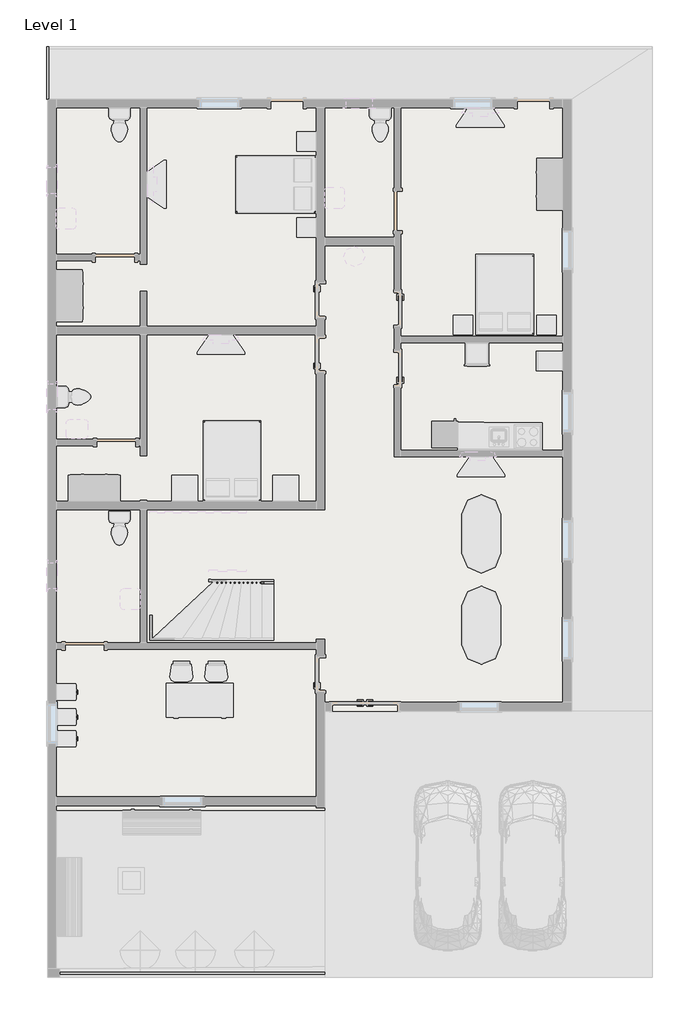
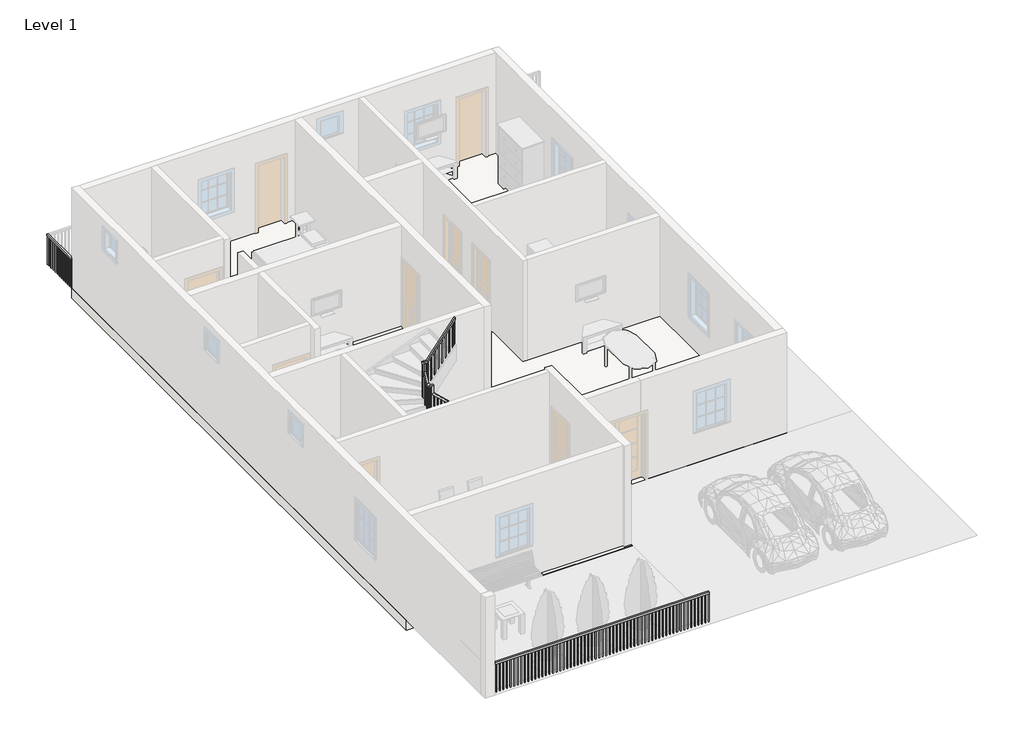
# One storey, part 2 of 4: 3 railings, 1 slab.
"""IFC4 building model written with IfcOpenShell, lengths in millimetres."""

from ifc_helpers import new_model, si_unit, frame, origin, origin_with_axes, place, context, project, spatial, polyline, outline, extrude, faceted_brep, element, save

model = new_model("IFC4")

# Units and contexts
model_context = context("Model", 3, world=origin())
ifc_project = project(units=[si_unit("LENGTHUNIT", "METRE", prefix="MILLI")], contexts=[model_context])

# Site, building, storey
site = spatial("IfcSite", under=ifc_project)
building = spatial("IfcBuilding", under=site)
storey = spatial("IfcBuildingStorey", under=building, Name="Level 1", Elevation=0.0)

# Railings
placement = place(None, origin())
element("IfcRailing", 1, ObjectType="Handrail - Rectangular", at=placement, inside=storey, context=model_context, shape_type="SolidModel", body=[
    faceted_brep([(-254.2696611, -2117.6011892, 992.3565828), (-254.2696611, -2117.6011892, 922.8758386), (-254.2696611, -2066.8011892, 922.8758386), (-254.2696611, -2066.8011892, 992.3565828), (-1705.801353, -2117.6011892, 2346.7909031), (-1756.601353, -2117.6011892, 2324.7119923), (-1756.601353, -2066.8011892, 2324.7119923), (-1705.801353, -2066.8011892, 2346.7909031), (-1705.801353, -2117.6011892, 2595.5341889), (-1756.601353, -2117.6011892, 2544.7341889), (-1756.601353, -2066.8011892, 2544.7341889), (-1705.801353, -2066.8011892, 2595.5341889), (-1832.801353, -2117.6011892, 2595.5341889), (-1832.801353, -2117.6011892, 2544.7341889), (-1782.001353, -2066.8011892, 2544.7341889), (-1782.001353, -2066.8011892, 2595.5341889), (-1832.801353, -1990.6011892, 2595.5341889), (-1832.801353, -1958.3784902, 2544.7341889), (-1782.001353, -1958.3784902, 2544.7341889), (-1782.001353, -1990.6011892, 2595.5341889), (-1832.801353, -1863.6011892, 2865.109353), (-1832.801353, -1812.8011892, 2853.7422582), (-1782.001353, -1812.8011892, 2853.7422582), (-1782.001353, -1863.6011892, 2865.109353), (-1832.801353, -1863.6011892, 3111.7887973), (-1832.801353, -1812.8011892, 3060.9887973), (-1782.001353, -1812.8011892, 3060.9887973), (-1782.001353, -1863.6011892, 3111.7887973), (-1832.801353, -1736.6011892, 3111.7887973), (-1832.801353, -1736.6011892, 3060.9887973), (-1782.001353, -1787.4011892, 3060.9887973), (-1782.001353, -1787.4011892, 3111.7887973), (-1705.801353, -1736.6011892, 3111.7887973), (-1680.8879409, -1736.6011892, 3060.9887973), (-1680.8879409, -1787.4011892, 3060.9887973), (-1705.801353, -1787.4011892, 3111.7887973), (-898.8739925, -1736.6011892, 4153.8992053), (-898.8739925, -1787.4011892, 4153.8992053), (-898.8739925, -1787.4011892, 4070.9246536), (-898.8739925, -1736.6011892, 4070.9246536)], [[[0, 1, 2, 3]], [[1, 0, 4, 5]], [[2, 1, 5, 6]], [[3, 2, 6, 7]], [[0, 3, 7, 4]], [[5, 4, 8, 9]], [[6, 5, 9, 10]], [[7, 6, 10, 11]], [[4, 7, 11, 8]], [[9, 8, 12, 13]], [[10, 9, 13, 14]], [[11, 10, 14, 15]], [[8, 11, 15, 12]], [[13, 12, 16, 17]], [[14, 13, 17, 18]], [[15, 14, 18, 19]], [[12, 15, 19, 16]], [[17, 16, 20, 21]], [[18, 17, 21, 22]], [[19, 18, 22, 23]], [[16, 19, 23, 20]], [[21, 20, 24, 25]], [[22, 21, 25, 26]], [[23, 22, 26, 27]], [[20, 23, 27, 24]], [[25, 24, 28, 29]], [[26, 25, 29, 30]], [[27, 26, 30, 31]], [[24, 27, 31, 28]], [[29, 28, 32, 33]], [[30, 29, 33, 34]], [[31, 30, 34, 35]], [[28, 31, 35, 32]], [[36, 37, 38, 39]], [[33, 32, 36, 39]], [[34, 33, 39, 38]], [[35, 34, 38, 37]], [[32, 35, 37, 36]]]),
    extrude(outline(polyline([(4009.6944401, -946.2857967), (3985.0922216, -965.3357967), (2878.6666667, -965.3357967), (2878.6666667, -946.2857967), (4009.6944401, -946.2857967)])), frame((0.0, -1771.5261892, 0.0), z_axis=(0.0, 1.0, 0.0), x_axis=(0.0, 0.0, 1.0)), (0.0, 0.0, 1.0), 19.05),
    extrude(outline(polyline([(3878.4826079, -1047.8857967), (3853.8803893, -1066.9357967), (2878.6666667, -1066.9357967), (2878.6666667, -1047.8857967), (3878.4826079, -1047.8857967)])), frame((0.0, -1771.5261892, 0.0), z_axis=(0.0, 1.0, 0.0), x_axis=(0.0, 0.0, 1.0)), (0.0, 0.0, 1.0), 19.05),
    extrude(outline(polyline([(3747.2707757, -1149.4857967), (3722.6685571, -1168.5357967), (2878.6666667, -1168.5357967), (2878.6666667, -1149.4857967), (3747.2707757, -1149.4857967)])), frame((0.0, -1771.5261892, 0.0), z_axis=(0.0, 1.0, 0.0), x_axis=(0.0, 0.0, 1.0)), (0.0, 0.0, 1.0), 19.05),
    extrude(outline(polyline([(3616.0589434, -1251.0857967), (3591.4567249, -1270.1357967), (2709.3333333, -1270.1357967), (2709.3333333, -1251.0857967), (3616.0589434, -1251.0857967)])), frame((0.0, -1771.5261892, 0.0), z_axis=(0.0, 1.0, 0.0), x_axis=(0.0, 0.0, 1.0)), (0.0, 0.0, 1.0), 19.05),
    extrude(outline(polyline([(3484.8471112, -1352.6857967), (3460.2448926, -1371.7357967), (2709.3333333, -1371.7357967), (2709.3333333, -1352.6857967), (3484.8471112, -1352.6857967)])), frame((0.0, -1771.5261892, 0.0), z_axis=(0.0, 1.0, 0.0), x_axis=(0.0, 0.0, 1.0)), (0.0, 0.0, 1.0), 19.05),
    extrude(outline(polyline([(3353.6352789, -1454.2857967), (3329.0330604, -1473.3357967), (2540.0, -1473.3357967), (2540.0, -1454.2857967), (3353.6352789, -1454.2857967)])), frame((0.0, -1771.5261892, 0.0), z_axis=(0.0, 1.0, 0.0), x_axis=(0.0, 0.0, 1.0)), (0.0, 0.0, 1.0), 19.05),
    extrude(outline(polyline([(3222.4234467, -1555.8857967), (3197.8212281, -1574.9357967), (2370.6666667, -1574.9357967), (2370.6666667, -1555.8857967), (3222.4234467, -1555.8857967)])), frame((0.0, -1771.5261892, 0.0), z_axis=(0.0, 1.0, 0.0), x_axis=(0.0, 0.0, 1.0)), (0.0, 0.0, 1.0), 19.05),
    extrude(outline(polyline([(3091.2116145, -1657.4857967), (3066.6093959, -1676.5357967), (2201.3333333, -1676.5357967), (2201.3333333, -1657.4857967), (3091.2116145, -1657.4857967)])), frame((0.0, -1771.5261892, 0.0), z_axis=(0.0, 1.0, 0.0), x_axis=(0.0, 0.0, 1.0)), (0.0, 0.0, 1.0), 19.05),
    extrude(outline(polyline([(-1883.987563, 2702.6392786), (-1864.937563, 2743.0755532), (-1864.937563, 1862.6666667), (-1883.987563, 1862.6666667), (-1883.987563, 2702.6392786)])), frame((-1816.926353, 0.0, 0.0), z_axis=(1.0, 0.0, 0.0), x_axis=(0.0, 1.0, 0.0)), (0.0, 0.0, 1.0), 19.05),
    extrude(outline(polyline([(-1985.587563, 2486.9791473), (-1966.537563, 2527.415422), (-1966.537563, 1693.3333333), (-1985.587563, 1693.3333333), (-1985.587563, 2486.9791473)])), frame((-1816.926353, 0.0, 0.0), z_axis=(1.0, 0.0, 0.0), x_axis=(0.0, 1.0, 0.0)), (0.0, 0.0, 1.0), 19.05),
    extrude(outline(polyline([(2241.2393308, -1667.1446611), (2259.0150183, -1686.1946611), (1354.6666667, -1686.1946611), (1354.6666667, -1667.1446611), (2241.2393308, -1667.1446611)])), frame((0.0, -2101.7261892, 0.0), z_axis=(0.0, 1.0, 0.0), x_axis=(0.0, 0.0, 1.0)), (0.0, 0.0, 1.0), 19.05),
    extrude(outline(polyline([(2146.435664, -1565.5446611), (2164.2113515, -1584.5946611), (1185.3333333, -1584.5946611), (1185.3333333, -1565.5446611), (2146.435664, -1565.5446611)])), frame((0.0, -2101.7261892, 0.0), z_axis=(0.0, 1.0, 0.0), x_axis=(0.0, 0.0, 1.0)), (0.0, 0.0, 1.0), 19.05),
    extrude(outline(polyline([(2051.6319971, -1463.9446611), (2069.4076846, -1482.9946611), (1016.0, -1482.9946611), (1016.0, -1463.9446611), (2051.6319971, -1463.9446611)])), frame((0.0, -2101.7261892, 0.0), z_axis=(0.0, 1.0, 0.0), x_axis=(0.0, 0.0, 1.0)), (0.0, 0.0, 1.0), 19.05),
    extrude(outline(polyline([(1956.8283302, -1362.3446611), (1974.6040178, -1381.3946611), (1016.0, -1381.3946611), (1016.0, -1362.3446611), (1956.8283302, -1362.3446611)])), frame((0.0, -2101.7261892, 0.0), z_axis=(0.0, 1.0, 0.0), x_axis=(0.0, 0.0, 1.0)), (0.0, 0.0, 1.0), 19.05),
    extrude(outline(polyline([(1862.0246634, -1260.7446611), (1879.8003509, -1279.7946611), (846.6666667, -1279.7946611), (846.6666667, -1260.7446611), (1862.0246634, -1260.7446611)])), frame((0.0, -2101.7261892, 0.0), z_axis=(0.0, 1.0, 0.0), x_axis=(0.0, 0.0, 1.0)), (0.0, 0.0, 1.0), 19.05),
    extrude(outline(polyline([(1767.2209965, -1159.1446611), (1784.9966841, -1178.1946611), (677.3333333, -1178.1946611), (677.3333333, -1159.1446611), (1767.2209965, -1159.1446611)])), frame((0.0, -2101.7261892, 0.0), z_axis=(0.0, 1.0, 0.0), x_axis=(0.0, 0.0, 1.0)), (0.0, 0.0, 1.0), 19.05),
    extrude(outline(polyline([(1672.4173297, -1057.5446611), (1690.1930172, -1076.5946611), (677.3333333, -1076.5946611), (677.3333333, -1057.5446611), (1672.4173297, -1057.5446611)])), frame((0.0, -2101.7261892, 0.0), z_axis=(0.0, 1.0, 0.0), x_axis=(0.0, 0.0, 1.0)), (0.0, 0.0, 1.0), 19.05),
    extrude(outline(polyline([(1577.6136628, -955.9446611), (1595.3893504, -974.9946611), (508.0, -974.9946611), (508.0, -955.9446611), (1577.6136628, -955.9446611)])), frame((0.0, -2101.7261892, 0.0), z_axis=(0.0, 1.0, 0.0), x_axis=(0.0, 0.0, 1.0)), (0.0, 0.0, 1.0), 19.05),
    extrude(outline(polyline([(1482.809996, -854.3446611), (1500.5856835, -873.3946611), (508.0, -873.3946611), (508.0, -854.3446611), (1482.809996, -854.3446611)])), frame((0.0, -2101.7261892, 0.0), z_axis=(0.0, 1.0, 0.0), x_axis=(0.0, 0.0, 1.0)), (0.0, 0.0, 1.0), 19.05),
    extrude(outline(polyline([(1388.0063291, -752.7446611), (1405.7820167, -771.7946611), (338.6666667, -771.7946611), (338.6666667, -752.7446611), (1388.0063291, -752.7446611)])), frame((0.0, -2101.7261892, 0.0), z_axis=(0.0, 1.0, 0.0), x_axis=(0.0, 0.0, 1.0)), (0.0, 0.0, 1.0), 19.05),
    extrude(outline(polyline([(1293.2026623, -651.1446611), (1310.9783498, -670.1946611), (338.6666667, -670.1946611), (338.6666667, -651.1446611), (1293.2026623, -651.1446611)])), frame((0.0, -2101.7261892, 0.0), z_axis=(0.0, 1.0, 0.0), x_axis=(0.0, 0.0, 1.0)), (0.0, 0.0, 1.0), 19.05),
    extrude(outline(polyline([(1198.3989954, -549.5446611), (1216.174683, -568.5946611), (338.6666667, -568.5946611), (338.6666667, -549.5446611), (1198.3989954, -549.5446611)])), frame((0.0, -2101.7261892, 0.0), z_axis=(0.0, 1.0, 0.0), x_axis=(0.0, 0.0, 1.0)), (0.0, 0.0, 1.0), 19.05),
    extrude(outline(polyline([(1103.5953286, -447.9446611), (1121.3710161, -466.9946611), (169.3333333, -466.9946611), (169.3333333, -447.9446611), (1103.5953286, -447.9446611)])), frame((0.0, -2101.7261892, 0.0), z_axis=(0.0, 1.0, 0.0), x_axis=(0.0, 0.0, 1.0)), (0.0, 0.0, 1.0), 19.05),
    extrude(outline(polyline([(1008.7916617, -346.3446611), (1026.5673493, -365.3946611), (169.3333333, -365.3946611), (169.3333333, -346.3446611), (1008.7916617, -346.3446611)])), frame((0.0, -2101.7261892, 0.0), z_axis=(0.0, 1.0, 0.0), x_axis=(0.0, 0.0, 1.0)), (0.0, 0.0, 1.0), 19.05),
    extrude(outline(polyline([(-1778.1357967, -1771.5261892), (-1778.1357967, -1752.4761892), (-1759.0857967, -1752.4761892), (-1759.0857967, -1771.5261892), (-1778.1357967, -1771.5261892)])), frame((0.0, 0.0, 2032.0), z_axis=(0.0, 0.0, 1.0), x_axis=(1.0, 0.0, 0.0)), (0.0, 0.0, 1.0), 1028.9887973),
    extrude(outline(polyline([(-1797.876353, -1771.5261892), (-1816.926353, -1771.5261892), (-1816.926353, -1752.4761892), (-1797.876353, -1752.4761892), (-1797.876353, -1771.5261892)])), frame((0.0, 0.0, 2032.0), z_axis=(0.0, 0.0, 1.0), x_axis=(1.0, 0.0, 0.0)), (0.0, 0.0, 1.0), 1028.9887973),
    extrude(outline(polyline([(-1797.876353, -1795.1271206), (-1816.926353, -1795.1271206), (-1816.926353, -1776.0771206), (-1797.876353, -1776.0771206), (-1797.876353, -1795.1271206)])), frame((0.0, 0.0, 2032.0), z_axis=(0.0, 0.0, 1.0), x_axis=(1.0, 0.0, 0.0)), (0.0, 0.0, 1.0), 1028.9887973),
    extrude(outline(polyline([(-1797.876353, -2087.187563), (-1816.926353, -2087.187563), (-1816.926353, -2068.137563), (-1797.876353, -2068.137563), (-1797.876353, -2087.187563)])), frame((0.0, 0.0, 1524.0), z_axis=(0.0, 0.0, 1.0), x_axis=(1.0, 0.0, 0.0)), (0.0, 0.0, 1.0), 1020.7341889),
    extrude(outline(polyline([(-1797.876353, -2082.6761892), (-1797.876353, -2101.7261892), (-1816.926353, -2101.7261892), (-1816.926353, -2082.6761892), (-1797.876353, -2082.6761892)])), frame((0.0, 0.0, 1354.6666667), z_axis=(0.0, 0.0, 1.0), x_axis=(1.0, 0.0, 0.0)), (0.0, 0.0, 1.0), 1190.0675223),
    extrude(outline(polyline([(-1764.8037713, -2082.6761892), (-1764.8037713, -2101.7261892), (-1783.8537713, -2101.7261892), (-1783.8537713, -2082.6761892), (-1764.8037713, -2082.6761892)])), frame((0.0, 0.0, 1354.6666667), z_axis=(0.0, 0.0, 1.0), x_axis=(1.0, 0.0, 0.0)), (0.0, 0.0, 1.0), 1190.0675223),
    extrude(outline(polyline([(4070.9246536, -898.8739925), (4046.3224351, -917.9239925), (2878.6666667, -917.9239925), (2878.6666667, -898.8739925), (4070.9246536, -898.8739925)])), frame((0.0, -1771.5261892, 0.0), z_axis=(0.0, 1.0, 0.0), x_axis=(0.0, 0.0, 1.0)), (0.0, 0.0, 1.0), 19.05),
    extrude(outline(polyline([(922.8758386, -254.2696611), (940.6515262, -273.3196611), (169.3333333, -273.3196611), (169.3333333, -254.2696611), (922.8758386, -254.2696611)])), frame((0.0, -2101.7261892, 0.0), z_axis=(0.0, 1.0, 0.0), x_axis=(0.0, 0.0, 1.0)), (0.0, 0.0, 1.0), 19.05),
])
element("IfcRailing", 2, ObjectType="Handrail - Rectangular", at=placement, inside=storey, context=model_context, shape_type="SweptSolid", body=[
    extrude(outline(polyline([(-5515.801353, 9210.7988108), (-5566.601353, 9210.7988108), (-5566.601353, 10429.9988108), (-5515.801353, 10429.9988108), (-5515.801353, 9210.7988108)])), frame((0.0, 0.0, 863.6), z_axis=(0.0, 0.0, 1.0), x_axis=(1.0, 0.0, 0.0)), (0.0, 0.0, 1.0), 50.8),
    extrude(outline(polyline([(-5531.676353, 10318.8738108), (-5550.726353, 10318.8738108), (-5550.726353, 10337.9238108), (-5531.676353, 10337.9238108), (-5531.676353, 10318.8738108)])), origin_with_axes(), (0.0, 0.0, 1.0), 863.6),
    extrude(outline(polyline([(-5531.676353, 10217.2738108), (-5550.726353, 10217.2738108), (-5550.726353, 10236.3238108), (-5531.676353, 10236.3238108), (-5531.676353, 10217.2738108)])), origin_with_axes(), (0.0, 0.0, 1.0), 863.6),
    extrude(outline(polyline([(-5531.676353, 10115.6738108), (-5550.726353, 10115.6738108), (-5550.726353, 10134.7238108), (-5531.676353, 10134.7238108), (-5531.676353, 10115.6738108)])), origin_with_axes(), (0.0, 0.0, 1.0), 863.6),
    extrude(outline(polyline([(-5531.676353, 10014.0738108), (-5550.726353, 10014.0738108), (-5550.726353, 10033.1238108), (-5531.676353, 10033.1238108), (-5531.676353, 10014.0738108)])), origin_with_axes(), (0.0, 0.0, 1.0), 863.6),
    extrude(outline(polyline([(-5531.676353, 9912.4738108), (-5550.726353, 9912.4738108), (-5550.726353, 9931.5238108), (-5531.676353, 9931.5238108), (-5531.676353, 9912.4738108)])), origin_with_axes(), (0.0, 0.0, 1.0), 863.6),
    extrude(outline(polyline([(-5531.676353, 9810.8738108), (-5550.726353, 9810.8738108), (-5550.726353, 9829.9238108), (-5531.676353, 9829.9238108), (-5531.676353, 9810.8738108)])), origin_with_axes(), (0.0, 0.0, 1.0), 863.6),
    extrude(outline(polyline([(-5531.676353, 9709.2738108), (-5550.726353, 9709.2738108), (-5550.726353, 9728.3238108), (-5531.676353, 9728.3238108), (-5531.676353, 9709.2738108)])), origin_with_axes(), (0.0, 0.0, 1.0), 863.6),
    extrude(outline(polyline([(-5531.676353, 9607.6738108), (-5550.726353, 9607.6738108), (-5550.726353, 9626.7238108), (-5531.676353, 9626.7238108), (-5531.676353, 9607.6738108)])), origin_with_axes(), (0.0, 0.0, 1.0), 863.6),
    extrude(outline(polyline([(-5531.676353, 9506.0738108), (-5550.726353, 9506.0738108), (-5550.726353, 9525.1238108), (-5531.676353, 9525.1238108), (-5531.676353, 9506.0738108)])), origin_with_axes(), (0.0, 0.0, 1.0), 863.6),
    extrude(outline(polyline([(-5531.676353, 9404.4738108), (-5550.726353, 9404.4738108), (-5550.726353, 9423.5238108), (-5531.676353, 9423.5238108), (-5531.676353, 9404.4738108)])), origin_with_axes(), (0.0, 0.0, 1.0), 863.6),
    extrude(outline(polyline([(-5531.676353, 9302.8738108), (-5550.726353, 9302.8738108), (-5550.726353, 9321.9238108), (-5531.676353, 9321.9238108), (-5531.676353, 9302.8738108)])), origin_with_axes(), (0.0, 0.0, 1.0), 863.6),
    extrude(outline(polyline([(-5531.676353, 10410.9488108), (-5550.726353, 10410.9488108), (-5550.726353, 10429.9988108), (-5531.676353, 10429.9988108), (-5531.676353, 10410.9488108)])), origin_with_axes(), (0.0, 0.0, 1.0), 863.6),
    extrude(outline(polyline([(-5531.676353, 9210.7988108), (-5550.726353, 9210.7988108), (-5550.726353, 9229.8488108), (-5531.676353, 9229.8488108), (-5531.676353, 9210.7988108)])), origin_with_axes(), (0.0, 0.0, 1.0), 863.6),
])
element("IfcRailing", 3, ObjectType="Handrail - Rectangular", at=placement, inside=storey, context=model_context, shape_type="SweptSolid", body=[
    extrude(outline(polyline([(-5261.801353, -11236.2011892), (-5261.801353, -11185.4011892), (935.798647, -11185.4011892), (935.798647, -11236.2011892), (-5261.801353, -11236.2011892)])), frame((0.0, 0.0, 863.6), z_axis=(0.0, 0.0, 1.0), x_axis=(1.0, 0.0, 0.0)), (0.0, 0.0, 1.0), 50.8),
    extrude(outline(polyline([(824.673647, -11220.3261892), (824.673647, -11201.2761892), (843.723647, -11201.2761892), (843.723647, -11220.3261892), (824.673647, -11220.3261892)])), origin_with_axes(), (0.0, 0.0, 1.0), 863.6),
    extrude(outline(polyline([(723.073647, -11220.3261892), (723.073647, -11201.2761892), (742.123647, -11201.2761892), (742.123647, -11220.3261892), (723.073647, -11220.3261892)])), origin_with_axes(), (0.0, 0.0, 1.0), 863.6),
    extrude(outline(polyline([(621.473647, -11220.3261892), (621.473647, -11201.2761892), (640.523647, -11201.2761892), (640.523647, -11220.3261892), (621.473647, -11220.3261892)])), origin_with_axes(), (0.0, 0.0, 1.0), 863.6),
    extrude(outline(polyline([(519.873647, -11220.3261892), (519.873647, -11201.2761892), (538.923647, -11201.2761892), (538.923647, -11220.3261892), (519.873647, -11220.3261892)])), origin_with_axes(), (0.0, 0.0, 1.0), 863.6),
    extrude(outline(polyline([(418.273647, -11220.3261892), (418.273647, -11201.2761892), (437.323647, -11201.2761892), (437.323647, -11220.3261892), (418.273647, -11220.3261892)])), origin_with_axes(), (0.0, 0.0, 1.0), 863.6),
    extrude(outline(polyline([(316.673647, -11220.3261892), (316.673647, -11201.2761892), (335.723647, -11201.2761892), (335.723647, -11220.3261892), (316.673647, -11220.3261892)])), origin_with_axes(), (0.0, 0.0, 1.0), 863.6),
    extrude(outline(polyline([(215.073647, -11220.3261892), (215.073647, -11201.2761892), (234.123647, -11201.2761892), (234.123647, -11220.3261892), (215.073647, -11220.3261892)])), origin_with_axes(), (0.0, 0.0, 1.0), 863.6),
    extrude(outline(polyline([(113.473647, -11220.3261892), (113.473647, -11201.2761892), (132.523647, -11201.2761892), (132.523647, -11220.3261892), (113.473647, -11220.3261892)])), origin_with_axes(), (0.0, 0.0, 1.0), 863.6),
    extrude(outline(polyline([(11.873647, -11220.3261892), (11.873647, -11201.2761892), (30.923647, -11201.2761892), (30.923647, -11220.3261892), (11.873647, -11220.3261892)])), origin_with_axes(), (0.0, 0.0, 1.0), 863.6),
    extrude(outline(polyline([(-89.726353, -11220.3261892), (-89.726353, -11201.2761892), (-70.676353, -11201.2761892), (-70.676353, -11220.3261892), (-89.726353, -11220.3261892)])), origin_with_axes(), (0.0, 0.0, 1.0), 863.6),
    extrude(outline(polyline([(-191.326353, -11220.3261892), (-191.326353, -11201.2761892), (-172.276353, -11201.2761892), (-172.276353, -11220.3261892), (-191.326353, -11220.3261892)])), origin_with_axes(), (0.0, 0.0, 1.0), 863.6),
    extrude(outline(polyline([(-292.926353, -11220.3261892), (-292.926353, -11201.2761892), (-273.876353, -11201.2761892), (-273.876353, -11220.3261892), (-292.926353, -11220.3261892)])), origin_with_axes(), (0.0, 0.0, 1.0), 863.6),
    extrude(outline(polyline([(-394.526353, -11220.3261892), (-394.526353, -11201.2761892), (-375.476353, -11201.2761892), (-375.476353, -11220.3261892), (-394.526353, -11220.3261892)])), origin_with_axes(), (0.0, 0.0, 1.0), 863.6),
    extrude(outline(polyline([(-496.126353, -11220.3261892), (-496.126353, -11201.2761892), (-477.076353, -11201.2761892), (-477.076353, -11220.3261892), (-496.126353, -11220.3261892)])), origin_with_axes(), (0.0, 0.0, 1.0), 863.6),
    extrude(outline(polyline([(-597.726353, -11220.3261892), (-597.726353, -11201.2761892), (-578.676353, -11201.2761892), (-578.676353, -11220.3261892), (-597.726353, -11220.3261892)])), origin_with_axes(), (0.0, 0.0, 1.0), 863.6),
    extrude(outline(polyline([(-699.326353, -11220.3261892), (-699.326353, -11201.2761892), (-680.276353, -11201.2761892), (-680.276353, -11220.3261892), (-699.326353, -11220.3261892)])), origin_with_axes(), (0.0, 0.0, 1.0), 863.6),
    extrude(outline(polyline([(-800.926353, -11220.3261892), (-800.926353, -11201.2761892), (-781.876353, -11201.2761892), (-781.876353, -11220.3261892), (-800.926353, -11220.3261892)])), origin_with_axes(), (0.0, 0.0, 1.0), 863.6),
    extrude(outline(polyline([(-902.526353, -11220.3261892), (-902.526353, -11201.2761892), (-883.476353, -11201.2761892), (-883.476353, -11220.3261892), (-902.526353, -11220.3261892)])), origin_with_axes(), (0.0, 0.0, 1.0), 863.6),
    extrude(outline(polyline([(-1004.126353, -11220.3261892), (-1004.126353, -11201.2761892), (-985.076353, -11201.2761892), (-985.076353, -11220.3261892), (-1004.126353, -11220.3261892)])), origin_with_axes(), (0.0, 0.0, 1.0), 863.6),
    extrude(outline(polyline([(-1105.726353, -11220.3261892), (-1105.726353, -11201.2761892), (-1086.676353, -11201.2761892), (-1086.676353, -11220.3261892), (-1105.726353, -11220.3261892)])), origin_with_axes(), (0.0, 0.0, 1.0), 863.6),
    extrude(outline(polyline([(-1207.326353, -11220.3261892), (-1207.326353, -11201.2761892), (-1188.276353, -11201.2761892), (-1188.276353, -11220.3261892), (-1207.326353, -11220.3261892)])), origin_with_axes(), (0.0, 0.0, 1.0), 863.6),
    extrude(outline(polyline([(-1308.926353, -11220.3261892), (-1308.926353, -11201.2761892), (-1289.876353, -11201.2761892), (-1289.876353, -11220.3261892), (-1308.926353, -11220.3261892)])), origin_with_axes(), (0.0, 0.0, 1.0), 863.6),
    extrude(outline(polyline([(-1410.526353, -11220.3261892), (-1410.526353, -11201.2761892), (-1391.476353, -11201.2761892), (-1391.476353, -11220.3261892), (-1410.526353, -11220.3261892)])), origin_with_axes(), (0.0, 0.0, 1.0), 863.6),
    extrude(outline(polyline([(-1512.126353, -11220.3261892), (-1512.126353, -11201.2761892), (-1493.076353, -11201.2761892), (-1493.076353, -11220.3261892), (-1512.126353, -11220.3261892)])), origin_with_axes(), (0.0, 0.0, 1.0), 863.6),
    extrude(outline(polyline([(-1613.726353, -11220.3261892), (-1613.726353, -11201.2761892), (-1594.676353, -11201.2761892), (-1594.676353, -11220.3261892), (-1613.726353, -11220.3261892)])), origin_with_axes(), (0.0, 0.0, 1.0), 863.6),
    extrude(outline(polyline([(-1715.326353, -11220.3261892), (-1715.326353, -11201.2761892), (-1696.276353, -11201.2761892), (-1696.276353, -11220.3261892), (-1715.326353, -11220.3261892)])), origin_with_axes(), (0.0, 0.0, 1.0), 863.6),
    extrude(outline(polyline([(-1816.926353, -11220.3261892), (-1816.926353, -11201.2761892), (-1797.876353, -11201.2761892), (-1797.876353, -11220.3261892), (-1816.926353, -11220.3261892)])), origin_with_axes(), (0.0, 0.0, 1.0), 863.6),
    extrude(outline(polyline([(-1918.526353, -11220.3261892), (-1918.526353, -11201.2761892), (-1899.476353, -11201.2761892), (-1899.476353, -11220.3261892), (-1918.526353, -11220.3261892)])), origin_with_axes(), (0.0, 0.0, 1.0), 863.6),
    extrude(outline(polyline([(-2020.126353, -11220.3261892), (-2020.126353, -11201.2761892), (-2001.076353, -11201.2761892), (-2001.076353, -11220.3261892), (-2020.126353, -11220.3261892)])), origin_with_axes(), (0.0, 0.0, 1.0), 863.6),
    extrude(outline(polyline([(-2121.726353, -11220.3261892), (-2121.726353, -11201.2761892), (-2102.676353, -11201.2761892), (-2102.676353, -11220.3261892), (-2121.726353, -11220.3261892)])), origin_with_axes(), (0.0, 0.0, 1.0), 863.6),
    extrude(outline(polyline([(-2223.326353, -11220.3261892), (-2223.326353, -11201.2761892), (-2204.276353, -11201.2761892), (-2204.276353, -11220.3261892), (-2223.326353, -11220.3261892)])), origin_with_axes(), (0.0, 0.0, 1.0), 863.6),
    extrude(outline(polyline([(-2324.926353, -11220.3261892), (-2324.926353, -11201.2761892), (-2305.876353, -11201.2761892), (-2305.876353, -11220.3261892), (-2324.926353, -11220.3261892)])), origin_with_axes(), (0.0, 0.0, 1.0), 863.6),
    extrude(outline(polyline([(-2426.526353, -11220.3261892), (-2426.526353, -11201.2761892), (-2407.476353, -11201.2761892), (-2407.476353, -11220.3261892), (-2426.526353, -11220.3261892)])), origin_with_axes(), (0.0, 0.0, 1.0), 863.6),
    extrude(outline(polyline([(-2528.126353, -11220.3261892), (-2528.126353, -11201.2761892), (-2509.076353, -11201.2761892), (-2509.076353, -11220.3261892), (-2528.126353, -11220.3261892)])), origin_with_axes(), (0.0, 0.0, 1.0), 863.6),
    extrude(outline(polyline([(-2629.726353, -11220.3261892), (-2629.726353, -11201.2761892), (-2610.676353, -11201.2761892), (-2610.676353, -11220.3261892), (-2629.726353, -11220.3261892)])), origin_with_axes(), (0.0, 0.0, 1.0), 863.6),
    extrude(outline(polyline([(-2731.326353, -11220.3261892), (-2731.326353, -11201.2761892), (-2712.276353, -11201.2761892), (-2712.276353, -11220.3261892), (-2731.326353, -11220.3261892)])), origin_with_axes(), (0.0, 0.0, 1.0), 863.6),
    extrude(outline(polyline([(-2832.926353, -11220.3261892), (-2832.926353, -11201.2761892), (-2813.876353, -11201.2761892), (-2813.876353, -11220.3261892), (-2832.926353, -11220.3261892)])), origin_with_axes(), (0.0, 0.0, 1.0), 863.6),
    extrude(outline(polyline([(-2934.526353, -11220.3261892), (-2934.526353, -11201.2761892), (-2915.476353, -11201.2761892), (-2915.476353, -11220.3261892), (-2934.526353, -11220.3261892)])), origin_with_axes(), (0.0, 0.0, 1.0), 863.6),
    extrude(outline(polyline([(-3036.126353, -11220.3261892), (-3036.126353, -11201.2761892), (-3017.076353, -11201.2761892), (-3017.076353, -11220.3261892), (-3036.126353, -11220.3261892)])), origin_with_axes(), (0.0, 0.0, 1.0), 863.6),
    extrude(outline(polyline([(-3137.726353, -11220.3261892), (-3137.726353, -11201.2761892), (-3118.676353, -11201.2761892), (-3118.676353, -11220.3261892), (-3137.726353, -11220.3261892)])), origin_with_axes(), (0.0, 0.0, 1.0), 863.6),
    extrude(outline(polyline([(-3239.326353, -11220.3261892), (-3239.326353, -11201.2761892), (-3220.276353, -11201.2761892), (-3220.276353, -11220.3261892), (-3239.326353, -11220.3261892)])), origin_with_axes(), (0.0, 0.0, 1.0), 863.6),
    extrude(outline(polyline([(-3340.926353, -11220.3261892), (-3340.926353, -11201.2761892), (-3321.876353, -11201.2761892), (-3321.876353, -11220.3261892), (-3340.926353, -11220.3261892)])), origin_with_axes(), (0.0, 0.0, 1.0), 863.6),
    extrude(outline(polyline([(-3442.526353, -11220.3261892), (-3442.526353, -11201.2761892), (-3423.476353, -11201.2761892), (-3423.476353, -11220.3261892), (-3442.526353, -11220.3261892)])), origin_with_axes(), (0.0, 0.0, 1.0), 863.6),
    extrude(outline(polyline([(-3544.126353, -11220.3261892), (-3544.126353, -11201.2761892), (-3525.076353, -11201.2761892), (-3525.076353, -11220.3261892), (-3544.126353, -11220.3261892)])), origin_with_axes(), (0.0, 0.0, 1.0), 863.6),
    extrude(outline(polyline([(-3645.726353, -11220.3261892), (-3645.726353, -11201.2761892), (-3626.676353, -11201.2761892), (-3626.676353, -11220.3261892), (-3645.726353, -11220.3261892)])), origin_with_axes(), (0.0, 0.0, 1.0), 863.6),
    extrude(outline(polyline([(-3747.326353, -11220.3261892), (-3747.326353, -11201.2761892), (-3728.276353, -11201.2761892), (-3728.276353, -11220.3261892), (-3747.326353, -11220.3261892)])), origin_with_axes(), (0.0, 0.0, 1.0), 863.6),
    extrude(outline(polyline([(-3848.926353, -11220.3261892), (-3848.926353, -11201.2761892), (-3829.876353, -11201.2761892), (-3829.876353, -11220.3261892), (-3848.926353, -11220.3261892)])), origin_with_axes(), (0.0, 0.0, 1.0), 863.6),
    extrude(outline(polyline([(-3950.526353, -11220.3261892), (-3950.526353, -11201.2761892), (-3931.476353, -11201.2761892), (-3931.476353, -11220.3261892), (-3950.526353, -11220.3261892)])), origin_with_axes(), (0.0, 0.0, 1.0), 863.6),
    extrude(outline(polyline([(-4052.126353, -11220.3261892), (-4052.126353, -11201.2761892), (-4033.076353, -11201.2761892), (-4033.076353, -11220.3261892), (-4052.126353, -11220.3261892)])), origin_with_axes(), (0.0, 0.0, 1.0), 863.6),
    extrude(outline(polyline([(-4153.726353, -11220.3261892), (-4153.726353, -11201.2761892), (-4134.676353, -11201.2761892), (-4134.676353, -11220.3261892), (-4153.726353, -11220.3261892)])), origin_with_axes(), (0.0, 0.0, 1.0), 863.6),
    extrude(outline(polyline([(-4255.326353, -11220.3261892), (-4255.326353, -11201.2761892), (-4236.276353, -11201.2761892), (-4236.276353, -11220.3261892), (-4255.326353, -11220.3261892)])), origin_with_axes(), (0.0, 0.0, 1.0), 863.6),
    extrude(outline(polyline([(-4356.926353, -11220.3261892), (-4356.926353, -11201.2761892), (-4337.876353, -11201.2761892), (-4337.876353, -11220.3261892), (-4356.926353, -11220.3261892)])), origin_with_axes(), (0.0, 0.0, 1.0), 863.6),
    extrude(outline(polyline([(-4458.526353, -11220.3261892), (-4458.526353, -11201.2761892), (-4439.476353, -11201.2761892), (-4439.476353, -11220.3261892), (-4458.526353, -11220.3261892)])), origin_with_axes(), (0.0, 0.0, 1.0), 863.6),
    extrude(outline(polyline([(-4560.126353, -11220.3261892), (-4560.126353, -11201.2761892), (-4541.076353, -11201.2761892), (-4541.076353, -11220.3261892), (-4560.126353, -11220.3261892)])), origin_with_axes(), (0.0, 0.0, 1.0), 863.6),
    extrude(outline(polyline([(-4661.726353, -11220.3261892), (-4661.726353, -11201.2761892), (-4642.676353, -11201.2761892), (-4642.676353, -11220.3261892), (-4661.726353, -11220.3261892)])), origin_with_axes(), (0.0, 0.0, 1.0), 863.6),
    extrude(outline(polyline([(-4763.326353, -11220.3261892), (-4763.326353, -11201.2761892), (-4744.276353, -11201.2761892), (-4744.276353, -11220.3261892), (-4763.326353, -11220.3261892)])), origin_with_axes(), (0.0, 0.0, 1.0), 863.6),
    extrude(outline(polyline([(-4864.926353, -11220.3261892), (-4864.926353, -11201.2761892), (-4845.876353, -11201.2761892), (-4845.876353, -11220.3261892), (-4864.926353, -11220.3261892)])), origin_with_axes(), (0.0, 0.0, 1.0), 863.6),
    extrude(outline(polyline([(-4966.526353, -11220.3261892), (-4966.526353, -11201.2761892), (-4947.476353, -11201.2761892), (-4947.476353, -11220.3261892), (-4966.526353, -11220.3261892)])), origin_with_axes(), (0.0, 0.0, 1.0), 863.6),
    extrude(outline(polyline([(-5068.126353, -11220.3261892), (-5068.126353, -11201.2761892), (-5049.076353, -11201.2761892), (-5049.076353, -11220.3261892), (-5068.126353, -11220.3261892)])), origin_with_axes(), (0.0, 0.0, 1.0), 863.6),
    extrude(outline(polyline([(-5169.726353, -11220.3261892), (-5169.726353, -11201.2761892), (-5150.676353, -11201.2761892), (-5150.676353, -11220.3261892), (-5169.726353, -11220.3261892)])), origin_with_axes(), (0.0, 0.0, 1.0), 863.6),
    extrude(outline(polyline([(916.748647, -11220.3261892), (916.748647, -11201.2761892), (935.798647, -11201.2761892), (935.798647, -11220.3261892), (916.748647, -11220.3261892)])), origin_with_axes(), (0.0, 0.0, 1.0), 863.6),
    extrude(outline(polyline([(-5261.801353, -11220.3261892), (-5261.801353, -11201.2761892), (-5242.751353, -11201.2761892), (-5242.751353, -11220.3261892), (-5261.801353, -11220.3261892)])), origin_with_axes(), (0.0, 0.0, 1.0), 863.6),
])

# Slab
element("IfcSlab", 4, ObjectType="Generic - 12\"", at=placement, inside=storey, context=model_context, shape_type="SweptSolid", body=[
    extrude(outline(polyline([(6701.598647, 9210.7988108), (6701.598647, -5089.4011892), (935.798647, -5089.4011892), (935.798647, -7400.8011892), (-5541.201353, -7400.8011892), (-5541.201353, 9210.7988108), (6701.598647, 9210.7988108)])), frame((0.0, 0.0, -304.8), z_axis=(0.0, 0.0, 1.0), x_axis=(1.0, 0.0, 0.0)), (0.0, 0.0, 1.0), 304.8),
])

save(model, "model.ifc")

# Revit data of these elements
# Type "Handrail - Rectangular"
#   Assembly Code = "C2010400"
#   built-in parameter 1008612 = 0.0416667 (stored number, unit not read)
#   built-in parameter 1008611 = 0.0416667 (stored number, unit not read)
#   built-in parameter 1008609 = 0.333333 (stored number, unit not read)
#   built-in parameter 1008604 = 0.166667 (stored number, unit not read)
#   built-in parameter 1008603 = 0.166667 (stored number, unit not read)
#   Railing Height = 3' - 0"
#   built-in parameter 1008630 = 2
#   built-in parameter 1008610 = 2
#   built-in parameter 1008618 = Baluster - Square : 3/4"
# Type "Generic - 12\""
#   Assembly Code = "B1010"
#   Function = 0
#   Layers, outside or top first: 1' - 0" no material (function 1)
# Elements 1, 2, 3 (IfcRailing, "Handrail - Rectangular")
#   Phase Created = New Construction
# Element 4 (IfcSlab, "Generic - 12\"")
#   Height Offset From Level = 0' - 0"
#   Phase Created = New Construction
#   Materials on its faces: "Default Floor"
# Materials
#   "Default Floor": colour RGB 128 128 128, transparency 0
